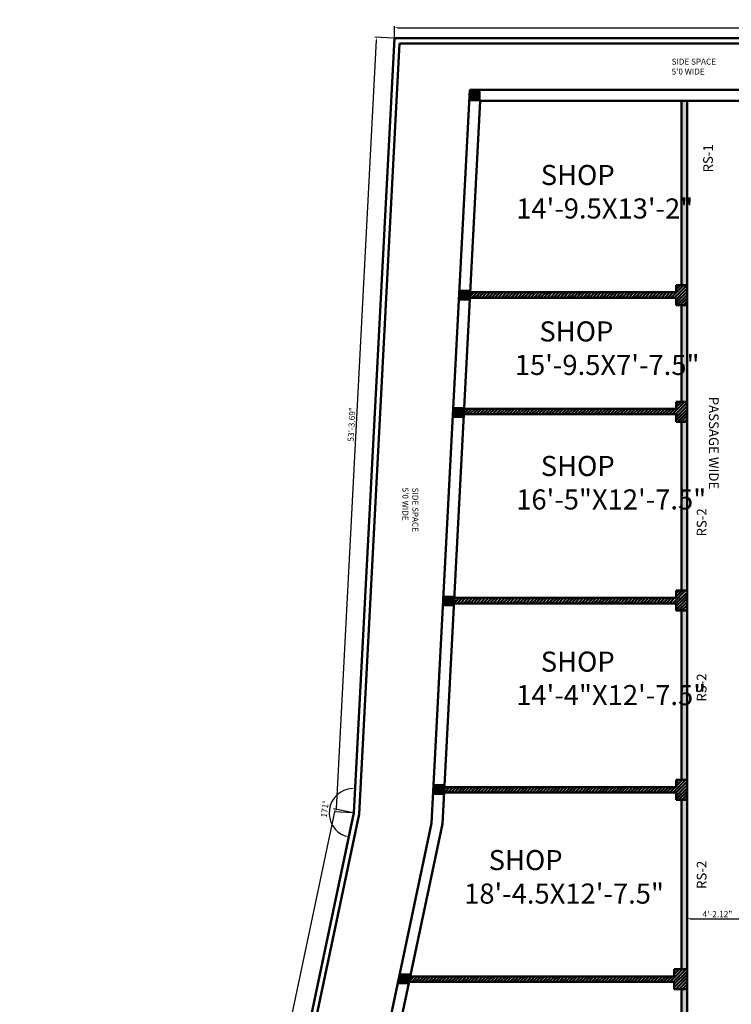
# Model space of a CAD drawing. Units: inches. Extents: x -2733 to 3435, y -338 to 1843.
# Tile 3 of 7: x -2733 to -2146, y 764 to 1575. Entities that reach past the tile are written whole.
import ezdxf

# ---------------------------------------------------------------- set-up
doc = ezdxf.new("R2010")
doc.units = ezdxf.units.IN
doc.header["$PDMODE"] = 34
for name, color, linetype, lineweight in [('A-ANNO-DIMS', 2, 'Continuous', 18), ('A-ANNO-TEXT', 7, 'Continuous', 18), ('A-AREA-IDEN', 3, 'Continuous', 18), ('A-COLS', 1, 'Continuous', 35), ('A-WALL', 7, 'Continuous', 50), ('A-WALL-PATT', 8, 'Continuous', 13)]:
    doc.layers.add(name, color=color, linetype=linetype, lineweight=lineweight)
doc.styles.get("Standard").update_dxf_attribs({"font": 'arial.ttf'})
doc.styles.add('YQ_DIM', font='SUPEROS.SHX', dxfattribs={"width": 0.8, "bigfont": 'HZDX.SHX'})
doc.dimstyles.new('ISO-25', dxfattribs={"dimtxt": 5, "dimasz": 2.5, "dimexe": 1.25, "dimexo": 0.625, "dimtad": 1, "dimlunit": 3, "dimtxsty": 'Standard', "dimcen": 2.5, "dimadec": 0, "dimazin": 0, "dimtfac": 1, "dimtmove": 0, "dimatfit": 3, "dimfxl": 1, "dimarcsym": 0})
pattern_1 = [(45, (-2862.9097, 0), (-1.3470384, 1.3470384), []), (45, (-2862.0116, 0), (-1.3470384, 1.3470384), [])]

# ---------------------------------------------------------------- blocks, each defined once
blk = doc.blocks.new('*D4')
at = {"layer": 'A-ANNO-DIMS', "color": 0, "lineweight": -2, "transparency": 16777216}
for p, q in [((-2424.19, 1560.16), (-2439.53, 1560.96)), ((-2438.42, 1558.4), (-2471.63, 924.58)), ((-2457.67, 921.35), (-2473.01, 922.15))]:
    blk.add_line(p, q, dxfattribs=at)
at = {"layer": 'A-ANNO-DIMS', "color": 0, "lineweight": 20, "transparency": 16777216}
for points in [[(-2438.83, 1558.42), (-2438, 1558.38), (-2438.28, 1560.9)], [(-2472.05, 924.6), (-2471.22, 924.56), (-2471.76, 922.08)]]:
    blk.add_solid(points, dxfattribs=at)
at = {"layer": 'Defpoints', "color": 0, "lineweight": 20, "transparency": 16777216}
for p in [(-2423.57, 1560.13), (-2471.76, 922.08), (-2457.05, 921.31)]:
    blk.add_point(p, dxfattribs=at)
at = {"layer": 'A-ANNO-DIMS', "color": 0, "transparency": 16777216, "insert": (-2458.2, 1241.66), "char_height": 5, "attachment_point": 5, "rotation": 87}
blk.add_mtext('53\'-3.69"', dxfattribs=at)
blk = doc.blocks.new('*D5')
at = {"layer": 'A-ANNO-DIMS', "color": 0, "lineweight": -2, "transparency": 16777216}
for p, q in [((-2472.99, 922.12), (-2730.86, -302.71)), ((-2457.66, 921.44), (-2473.7, 924.82)), ((-2716.56, -308.27), (-2732.6, -304.9))]:
    blk.add_line(p, q, dxfattribs=at)
at = {"layer": 'A-ANNO-DIMS', "color": 0, "lineweight": 20, "transparency": 16777216}
for points in [[(-2473.4, 922.2), (-2472.59, 922.03), (-2472.48, 924.56)], [(-2731.27, -302.62), (-2730.46, -302.79), (-2731.38, -305.15)]]:
    blk.add_solid(points, dxfattribs=at)
at = {"layer": 'Defpoints', "color": 0, "lineweight": 20, "transparency": 16777216}
for p in [(-2457.05, 921.31), (-2731.38, -305.15), (-2715.95, -308.4)]:
    blk.add_point(p, dxfattribs=at)
at = {"layer": 'A-ANNO-DIMS', "color": 0, "transparency": 16777216, "insert": (-2605.04, 310.36), "char_height": 5, "attachment_point": 5, "rotation": 78.11076}
blk.add_mtext('104\'-8.67"', dxfattribs=at)
blk = doc.blocks.new('*D9')
at = {"layer": 'A-ANNO-DIMS', "color": 0, "lineweight": -2, "transparency": 16777216}
for p, q in [((-2182.13, 829.34), (-2182.13, 835.34)), ((-2179.63, 834.09), (-2134.51, 834.09)), ((-2132.01, 829.34), (-2132.01, 835.34))]:
    blk.add_line(p, q, dxfattribs=at)
at = {"layer": 'A-ANNO-DIMS', "color": 0, "lineweight": 20, "transparency": 16777216}
for points in [[(-2179.63, 834.5), (-2179.63, 833.67), (-2182.13, 834.09)], [(-2134.51, 834.5), (-2134.51, 833.67), (-2132.01, 834.09)]]:
    blk.add_solid(points, dxfattribs=at)
at = {"layer": 'Defpoints', "color": 0, "lineweight": 20, "transparency": 16777216}
for p in [(-2182.13, 828.71), (-2132.01, 834.09), (-2132.01, 828.71)]:
    blk.add_point(p, dxfattribs=at)
at = {"layer": 'A-ANNO-DIMS', "color": 0, "transparency": 16777216, "insert": (-2157.07, 837.22), "char_height": 5, "attachment_point": 5}
blk.add_mtext('4\'-2.12"', dxfattribs=at)
blk = doc.blocks.new('*D13')
at = {"layer": 'A-ANNO-DIMS', "color": 0, "lineweight": -2, "transparency": 16777216}
for p, q in [((-2423.57, 1560.75), (-2423.57, 1570.04)), ((-2421.07, 1568.79), (-1749.07, 1568.79)), ((-1746.57, 1560.75), (-1746.57, 1570.04))]:
    blk.add_line(p, q, dxfattribs=at)
at = {"layer": 'A-ANNO-DIMS', "color": 0, "lineweight": 20, "transparency": 16777216}
for points in [[(-2421.07, 1569.21), (-2421.07, 1568.38), (-2423.57, 1568.79)], [(-1749.07, 1569.21), (-1749.07, 1568.38), (-1746.57, 1568.79)]]:
    blk.add_solid(points, dxfattribs=at)
at = {"layer": 'Defpoints', "color": 0, "lineweight": 20, "transparency": 16777216}
for p in [(-1746.57, 1568.79), (-2423.57, 1560.13), (-1746.57, 1560.13)]:
    blk.add_point(p, dxfattribs=at)
at = {"layer": 'A-ANNO-DIMS', "color": 0, "transparency": 16777216, "insert": (-2085.07, 1571.97), "char_height": 5, "attachment_point": 5}
blk.add_mtext('56\'-5"', dxfattribs=at)
blk = doc.blocks.new('*D22')
at = {"layer": 'A-ANNO-DIMS', "color": 0, "lineweight": -2, "transparency": 16777216}
blk.add_arc((-2457.05, 921.31), 20.29, 94.06404, 251.04672, dxfattribs=at)
at = {"layer": 'A-ANNO-DIMS', "color": 0, "lineweight": 20, "transparency": 16777216}
for points in [[(-2458.49, 941.97), (-2458.48, 941.14), (-2455.99, 941.58)], [(-2463.53, 902.53), (-2463.75, 901.72), (-2461.23, 901.46)]]:
    blk.add_solid(points, dxfattribs=at)
at = {"layer": 'Defpoints', "color": 0, "lineweight": 20, "transparency": 16777216}
for p in [(-2423.57, 1560.13), (-2473.47, 933.23), (-2457.05, 921.31), (-2457.05, 921.31), (-2718.34, -319.77)]:
    blk.add_point(p, dxfattribs=at)
at = {"layer": 'A-ANNO-DIMS', "color": 0, "transparency": 16777216, "insert": (-2480.28, 924.35), "char_height": 5, "attachment_point": 5, "rotation": 82.55538}
blk.add_mtext('171°', dxfattribs=at)

msp = doc.modelspace()

# ---------------------------------------------------------------- hatches: boundary and pattern name
at = {"layer": 'A-COLS'}
h = msp.add_hatch(color=256, dxfattribs=at)
h.dxf.hatch_style = 1
h.paths.add_polyline_path([(-2352.226, 1517), (-2361.226, 1517), (-2361.226, 1508), (-2352.226, 1508)])
h = msp.add_hatch(color=256, dxfattribs=at)
h.dxf.hatch_style = 1
h.paths.add_polyline_path([(-2361.289, 1352.746), (-2370.289, 1352.746), (-2370.289, 1343.746), (-2361.289, 1343.746)])
h = msp.add_hatch(color=256, dxfattribs=at)
h.dxf.hatch_style = 1
h.paths.add_polyline_path([(-2366.641, 1255.953), (-2375.641, 1255.953), (-2375.641, 1246.953), (-2366.641, 1246.953)])
h = msp.add_hatch(color=256, dxfattribs=at)
h.dxf.hatch_style = 1
h.paths.add_polyline_path([(-2374.671, 1100.549), (-2383.671, 1100.549), (-2383.671, 1091.549), (-2374.671, 1091.549)])
h = msp.add_hatch(color=256, dxfattribs=at)
h.dxf.hatch_style = 1
h.paths.add_polyline_path([(-2382.927, 945.146), (-2391.927, 945.146), (-2391.927, 936.146), (-2382.927, 936.146)])
h = msp.add_hatch(color=256, dxfattribs=at)
h.dxf.hatch_style = 1
h.paths.add_polyline_path([(-2410.943, 789.049), (-2419.943, 789.049), (-2419.943, 780.049), (-2410.943, 780.049)])
at = {"layer": 'A-WALL-PATT'}
h = msp.add_hatch(color=256, dxfattribs=at)
h.dxf.hatch_style = 1
h.paths.add_polyline_path([(-2182.126, 776.08), (-2186.626, 776.08), (-2186.626, 641.08), (-2182.126, 641.08)])
h.paths.add_polyline_path([(-2182.126, 932.085), (-2186.626, 932.085), (-2186.626, 792.58), (-2182.126, 792.58)])
h.paths.add_polyline_path([(-2182.126, 624.58), (-2186.626, 624.58), (-2186.626, 485.101), (-2182.126, 485.101)])
h.paths.add_polyline_path([(-2182.126, 468.606), (-2186.626, 468.606), (-2186.626, 341.08), (-2222.626, 305.08), (-2511.726, 305.08), (-2512.673, 300.58), (-2218.126, 300.58), (-2182.126, 336.58)])
h.paths.add_polyline_path([(-2182.126, 1088.154), (-2186.626, 1088.154), (-2186.626, 948.58), (-2182.126, 948.582)])
h.paths.add_polyline_path([(-2182.126, 1243.861), (-2186.626, 1243.861), (-2186.626, 1104.649), (-2182.126, 1104.649)])
h.paths.add_polyline_path([(-2182.126, 1340.024), (-2186.626, 1340.024), (-2186.626, 1260.356), (-2182.126, 1260.356)])
h.paths.add_polyline_path([(-2182.126, 1508.58), (-2186.626, 1508.58), (-2186.626, 1356.519), (-2182.126, 1356.519)])
h = msp.add_hatch(dxfattribs=at)
h.set_pattern_fill('ANSI32', color=256, scale=0.2)
h.set_pattern_definition(pattern_1)
h.paths.add_polyline_path([(-2182.126, 1356.519), (-2186.626, 1356.519), (-2191.126, 1356.519), (-2191.126, 1350.58), (-2360.949, 1350.58), (-2361.185, 1346.08), (-2191.126, 1346.08), (-2191.126, 1340.024), (-2186.626, 1340.024), (-2182.126, 1340.024)])
h.paths.add_polyline_path([(-2182.126, 1260.356), (-2186.626, 1260.356), (-2191.126, 1260.356), (-2191.126, 1254.58), (-2365.981, 1254.58), (-2366.216, 1250.08), (-2191.126, 1250.08), (-2191.126, 1243.861), (-2186.626, 1243.861), (-2182.126, 1243.861)])
h = msp.add_hatch(dxfattribs=at)
h.set_pattern_fill('ANSI32', color=256, scale=0.2)
h.set_pattern_definition(pattern_1)
h.paths.add_polyline_path([(-2182.126, 641.08), (-2186.626, 641.08), (-2186.626, 641.075), (-2191.126, 641.075), (-2191.126, 635.08), (-2442.281, 635.08), (-2443.228, 630.58), (-2191.126, 630.58), (-2191.126, 624.58), (-2186.626, 624.58), (-2182.126, 624.58)])
h.paths.add_polyline_path([(-2182.126, 1104.649), (-2191.126, 1104.649), (-2191.126, 1098.58), (-2374.156, 1098.58), (-2374.392, 1094.08), (-2191.126, 1094.08), (-2191.126, 1088.154), (-2182.126, 1088.154)])
h.paths.add_polyline_path([(-2182.126, 948.58), (-2186.626, 948.58), (-2191.126, 948.58), (-2191.126, 942.58), (-2382.332, 942.58), (-2382.556, 938.295), (-2191.126, 938.09), (-2191.126, 932.085), (-2186.626, 932.085), (-2182.126, 932.085)])
h.paths.add_polyline_path([(-2182.126, 485.101), (-2191.126, 485.101), (-2191.126, 479.08), (-2475.11, 479.08), (-2476.057, 474.58), (-2191.126, 474.58), (-2191.126, 468.606), (-2182.126, 468.606)])
h.paths.add_polyline_path([(-2182.126, 792.575), (-2192.673, 792.575), (-2192.673, 786.58), (-2410.4, 786.58), (-2411.347, 782.08), (-2192.673, 782.08), (-2192.673, 776.08), (-2186.626, 776.08), (-2182.126, 776.08)])

# ---------------------------------------------------------------- linework, layer by layer
at = {"layer": 'A-WALL'}
for p, q in [((-2457.047, 921.314), (-2423.568, 1560.127)), ((-2423.568, 1560.127), (-1746.569, 1560.127)), ((-2452.591, 920.356), (-2419.298, 1555.627)), ((-2419.298, 1555.627), (-1751.069, 1555.627)), ((-2392.898, 912.931), (-2361.21, 1517.58)), ((-2361.21, 1517.58), (-1811.069, 1517.58)), ((-2340.407, 1517.58), (-1811.069, 1517.58)), ((-2383.91, 912.46), (-2352.669, 1508.58)), ((-2352.669, 1508.58), (-1820.069, 1508.58)), ((-2348.399, 1508.58), (-1820.069, 1508.58)), ((-2186.626, 1508.58), (-2186.626, 1356.519)), ((-2182.126, 1508.58), (-2182.126, 336.58)), ((-2191.126, 1350.519), (-2191.126, 1356.519)), ((-2191.126, 1356.519), (-2186.626, 1356.519)), ((-2186.626, 1356.519), (-2182.126, 1356.519)), ((-2360.949, 1350.58), (-2191.126, 1350.58)), ((-2361.185, 1346.08), (-2191.126, 1346.08)), ((-2191.126, 1340.024), (-2191.126, 1346.08)), ((-2186.626, 1340.024), (-2191.126, 1340.024)), ((-2186.626, 1340.024), (-2186.626, 1260.356)), ((-2186.626, 1340.024), (-2182.126, 1340.024)), ((-2191.126, 1254.58), (-2191.126, 1260.356)), ((-2191.126, 1260.356), (-2186.626, 1260.356)), ((-2186.626, 1260.356), (-2182.126, 1260.356)), ((-2365.981, 1254.58), (-2191.126, 1254.58)), ((-2366.216, 1250.08), (-2191.126, 1250.08)), ((-2191.126, 1243.861), (-2191.126, 1250.08)), ((-2186.626, 1243.861), (-2191.126, 1243.861)), ((-2186.626, 1243.861), (-2186.626, 1104.58)), ((-2186.626, 1243.861), (-2182.126, 1243.861)), ((-2191.126, 1098.58), (-2191.126, 1104.649)), ((-2191.126, 1104.649), (-2182.126, 1104.649)), ((-2374.156, 1098.58), (-2191.126, 1098.58)), ((-2374.392, 1094.08), (-2191.126, 1094.08)), ((-2191.126, 1088.154), (-2191.126, 1094.159)), ((-2182.126, 1088.154), (-2191.126, 1088.154)), ((-2186.626, 1088.154), (-2186.626, 948.58)), ((-2382.328, 942.657), (-2191.126, 942.58)), ((-2191.126, 948.58), (-2186.626, 948.58)), ((-2191.126, 942.58), (-2191.126, 948.58)), ((-2186.626, 948.58), (-2182.126, 948.582)), ((-2382.556, 938.295), (-2191.126, 938.09)), ((-2191.126, 932.085), (-2191.126, 938.09)), ((-2186.626, 932.085), (-2191.126, 932.085)), ((-2186.626, 932.085), (-2186.626, 792.58)), ((-2186.626, 932.085), (-2182.126, 932.085)), ((-2718.342, -319.774), (-2457.047, 921.314)), ((-2711.812, -310.6), (-2452.644, 920.386)), ((-2452.644, 920.386), (-2452.59, 920.384)), ((-2528.543, 268.651), (-2392.898, 912.931)), ((-2518.444, 273.153), (-2383.91, 912.46)), ((-2192.673, 786.575), (-2192.673, 792.575)), ((-2192.673, 792.575), (-2182.126, 792.575)), ((-2186.626, 792.58), (-2182.126, 792.58)), ((-2411.25, 782.08), (-2192.673, 782.08)), ((-2410.302, 786.58), (-2192.673, 786.58)), ((-2192.673, 776.08), (-2192.673, 782.085)), ((-2186.626, 776.08), (-2192.673, 776.08)), ((-2186.626, 776.08), (-2186.626, 641.075)), ((-2186.626, 776.08), (-2182.126, 776.08))]:
    msp.add_line(p, q, dxfattribs=at)

# ---------------------------------------------------------------- texts
at = {"layer": 'A-ANNO-TEXT', "char_height": 8, "attachment_point": 1, "rotation": 90, "style": 'YQ_DIM'}
for s, insert in [('{\\fSwis721 BlkCn BT|b0|i0|c0|p34;RS-1}', (-2168.819, 1449.404)), ('{\\fSwis721 BlkCn BT|b0|i0|c0|p34;RS-2}', (-2174.09, 1149.247)), ('{\\fSwis721 BlkCn BT|b0|i0|c0|p34;RS-2}', (-2174.09, 1013.043)), ('{\\fSwis721 BlkCn BT|b0|i0|c0|p34;RS-2}', (-2174.09, 858.608))]:
    msp.add_mtext_dynamic_manual_height_columns(s, width=14.9584, gutter_width=12.5, heights=[0], dxfattribs=dict(at, insert=insert))
at = {"layer": 'A-AREA-IDEN', "attachment_point": 1, "style": 'YQ_DIM'}
for s, width, gutter_width, insert, char_height in [("{\\f@Arial Unicode MS|b0|i0|c134|p34;SIDE SPACE\\P5'0 WIDE}", 92.43125, 24.565, (-2194.833, 1543.248), 4.91305), ('{\\f@SimSun|b1|i0|c0|p2; \\f@Arial Unicode MS|b1|i0|c0|p34;   SHOP\\P14\'-9.5X13\'-2\\f@SimSun|b1|i0|c0|p2;"}', 128.94034, 26.518, (-2323.043, 1455.611), 16.56819), ('{\\f@SimSun|b1|i0|c0|p2; \\f@Arial Unicode MS|b1|i0|c0|p34;   SHOP\\P15\'-9.5X7\'-7.5\\f@SimSun|b1|i0|c0|p2;"}', 128.94034, 26.518, (-2324.17, 1326.616), 16.56819), ('{\\f@SimSun|b1|i0|c0|p2; \\f@Arial Unicode MS|b1|i0|c0|p34;   SHOP\\P16\'-5"X12\'-7.5\\f@SimSun|b1|i0|c0|p2;"}', 128.94034, 26.518, (-2323.043, 1215.685), 16.56819), ('{\\f@SimSun|b1|i0|c0|p2; \\f@Arial Unicode MS|b1|i0|c0|p34;   SHOP\\P14\'-4"X12\'-7.5\\f@SimSun|b1|i0|c0|p2;"}', 128.94034, 26.518, (-2323.043, 1054.363), 16.56819), ('{\\f@SimSun|b1|i0|c0|p2; \\f@Arial Unicode MS|b1|i0|c0|p34;   SHOP\\P18\'-4.5X12\'-7.5\\f@SimSun|b1|i0|c0|p2;"}', 128.94034, 26.518, (-2366.027, 890.727), 16.56819)]:
    msp.add_mtext_dynamic_manual_height_columns(s, width=width, gutter_width=gutter_width, heights=[0], dxfattribs=dict(at, insert=insert, char_height=char_height))
at = {"layer": 'A-AREA-IDEN', "attachment_point": 1, "rotation": 270, "style": 'YQ_DIM'}
for s, width, gutter_width, insert, char_height in [('\\pxsm2;{\\f@Microsoft YaHei|b0|i0|c0|p34;PASSAGE WIDE}', 84.49104, 12.5, (-2156.06, 1264.465), 8), ("{\\f@Arial Unicode MS|b0|i0|c134|p34;SIDE SPACE\\P5'0 WIDE}", 92.43125, 24.565, (-2403.812, 1189.548), 4.91305)]:
    msp.add_mtext_dynamic_manual_height_columns(s, width=width, gutter_width=gutter_width, heights=[0], dxfattribs=dict(at, insert=insert, char_height=char_height))

# ---------------------------------------------------------------- dimensions: what is measured, and where the dimension line sits
at = {"layer": 'A-ANNO-DIMS'}
for base, p1, p2, picture, middle in [((-1746.569, 1568.792), (-2423.568, 1560.127), (-1746.569, 1560.127), '*D13', (-2085.069, 1571.97)), ((-2132.006, 834.088), (-2182.126, 828.714), (-2132.006, 828.714), '*D9', (-2157.066, 837.223))]:
    dim = msp.add_linear_dim(base=base, p1=p1, p2=p2, dimstyle='ISO-25', override={"dimclrd": 0, "dimclre": 0, "dimclrt": 0}, dxfattribs=at)
    dim.commit()
    dim.dimension.update_dxf_attribs({"geometry": picture, "text_midpoint": middle})
dim = msp.add_angular_dim_2l(base=(-2473.47, 933.229), line1=((-2718.342, -319.774), (-2457.047, 921.314)), line2=((-2457.047, 921.314), (-2423.568, 1560.127)), dimstyle='ISO-25', override={"dimclrd": 0, "dimclre": 0, "dimclrt": 0}, dxfattribs=at)
dim.commit()
dim.dimension.update_dxf_attribs({"geometry": '*D22', "text_midpoint": (-2480.275, 924.349)})
for p1, p2, distance, picture, middle in [((-2423.568, 1560.127), (-2457.047, 921.314), -14.736, '*D4', (-2458.199, 1241.658)), ((-2457.047, 921.314), (-2715.948, -308.402), -15.77, '*D5', (-2605.039, 310.359))]:
    dim = msp.add_aligned_dim(p1=p1, p2=p2, distance=distance, dimstyle='ISO-25', override={"dimclrd": 0, "dimclre": 0, "dimclrt": 0}, dxfattribs=at)
    dim.commit()
    dim.dimension.update_dxf_attribs({"geometry": picture, "text_midpoint": middle})

doc.saveas('drawing.dxf')
